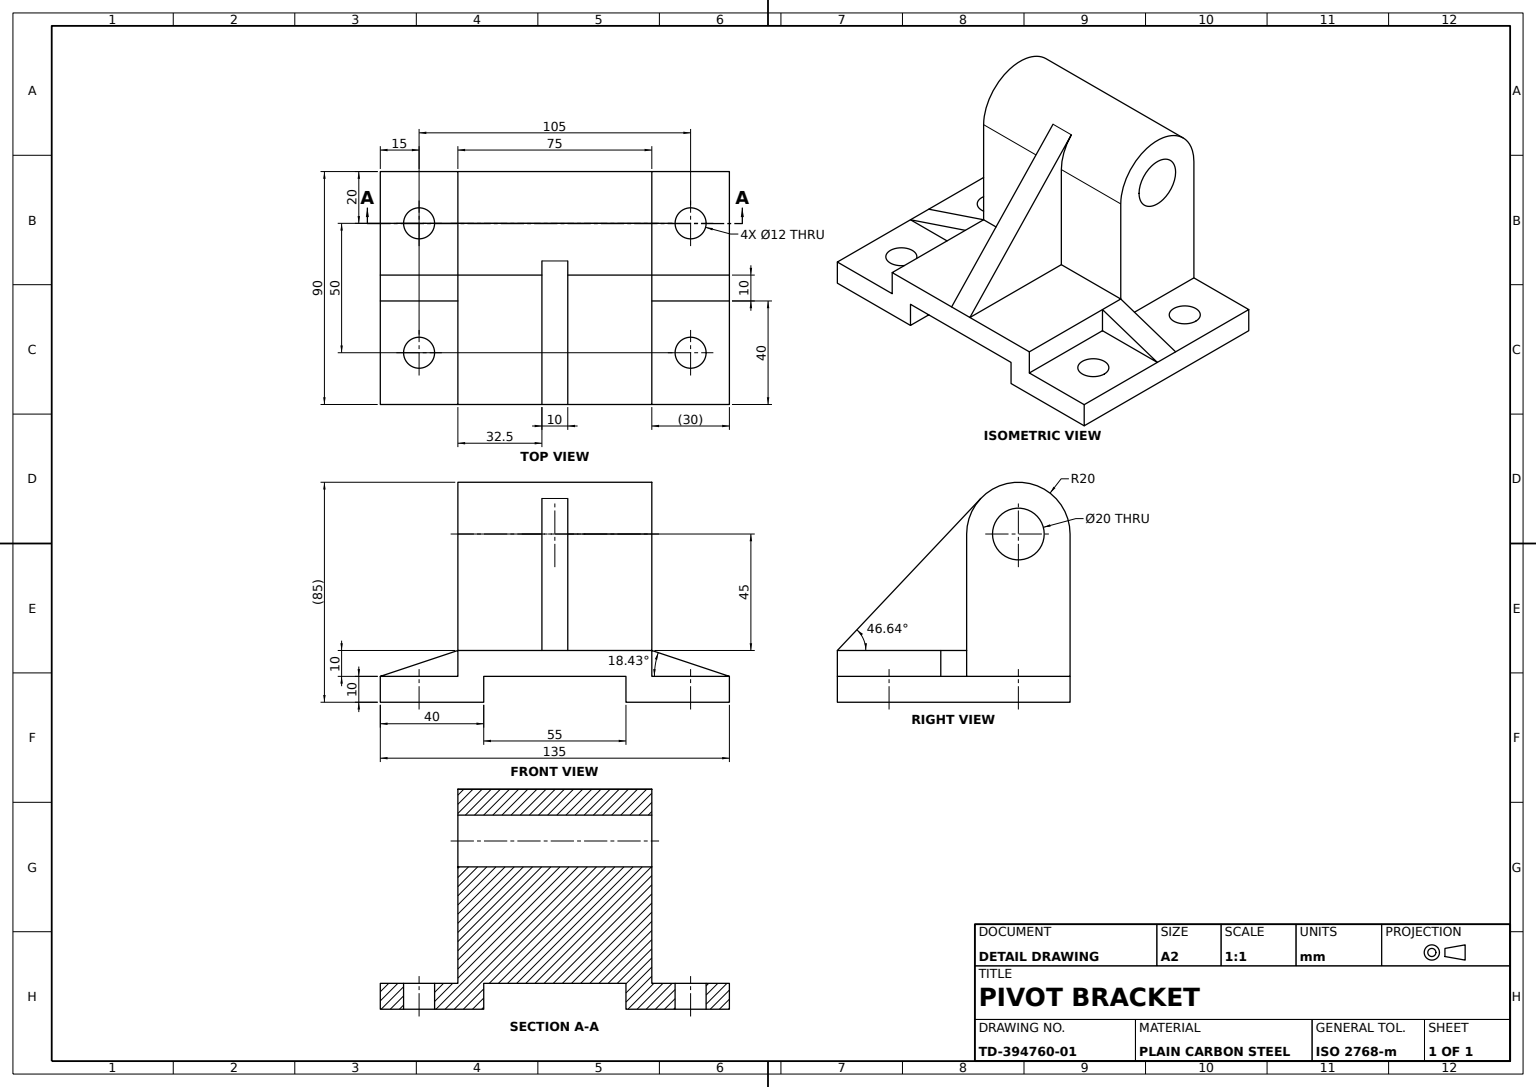
from build123d import *

# Parameters (mm, degrees)
BASE_PLATE_DEPTH            = 45
MOUNTING_HOLES_SKETCH_R     = 6
MOUNTING_HOLES_DEPTH        = 40
PIVOT_BOSS_PROFILE_R        = 10
PIVOT_BOSS_DEPTH            = 75
CENTER_GUSSET_RIB_REACH     = 119.5
CENTER_GUSSET_SKETCH_WALL_W = 317.777472108
CENTER_GUSSET_SKETCH_WALL_H = 10
SIDE_GUSSET_RIB_REACH       = 119.5
SIDE_GUSSET_SKETCH_WALL_W   = 268.622776602
SIDE_GUSSET_SKETCH_WALL_H   = 10


with BuildPart() as part:
    # Base Plate Profile → Base Plate (new, symmetric)
    with BuildSketch(Plane.XY):
        Polygon((-67.5, 0), (-27.5, 0), (-27.5, 10), (27.5, 10), (27.5, 0), (67.5, 0), (67.5, 10), (37.5, 10), (37.5, 20), (-37.5, 20), (-37.5, 10), (-67.5, 10), align=None)
    extrude(amount=BASE_PLATE_DEPTH, both=True)

    # Mounting Holes Sketch → Mounting Holes (cut)
    with BuildSketch(Plane(origin=(0, 10, 0), x_dir=(1, 0, 0), z_dir=(0, 1, 0))):
        with Locations(Location((52.5, -25, 0), (0, 0, 180))):
            Circle(MOUNTING_HOLES_SKETCH_R)
        with Locations(Location((52.5, 25, 0), (0, 0, 180))):
            Circle(MOUNTING_HOLES_SKETCH_R)
        with Locations(Location((-52.5, 25, 0), (0, 0, 270))):
            Circle(MOUNTING_HOLES_SKETCH_R)
        with Locations(Location((-52.5, -25, 0), (0, 0, 270))):
            Circle(MOUNTING_HOLES_SKETCH_R)
    extrude(amount=-MOUNTING_HOLES_DEPTH, mode=Mode.SUBTRACT)

    # Pivot Boss Profile → Pivot Boss (add)
    with BuildSketch(Plane(origin=(37.5, 0, 0), x_dir=(0, 0, -1), z_dir=(1, 0, 0))):
        with BuildLine():
            Line((45, 20), (5, 20))
            Line((5, 20), (5, 65))
            ThreePointArc((5, 65), (25, 85), (45, 65))
            Line((45, 65), (45, 20))
        make_face()
        with Locations((25, 65)):
            Circle(PIVOT_BOSS_PROFILE_R, mode=Mode.SUBTRACT)
    extrude(amount=-PIVOT_BOSS_DEPTH)

    # Center Gusset Sketch wall → Center Gusset Rib (add, up to next)
    with BuildSketch(Plane(origin=(0, 49.365592849, 17.270738259), x_dir=(0, -0.727073825966, 0.686559284837), z_dir=(0, -0.686559284837, -0.727073825966)), mode=Mode.PRIVATE) as center_gusset_rib_sk1:
        Rectangle(CENTER_GUSSET_SKETCH_WALL_W, CENTER_GUSSET_SKETCH_WALL_H)
    center_gusset_rib_tool1 = extrude(center_gusset_rib_sk1.sketch, amount=CENTER_GUSSET_RIB_REACH, mode=Mode.PRIVATE) - part.part
    add(center_gusset_rib_tool1.solids().sort_by_distance((0, 49.365592849, 17.270738259))[0])

    # Side Gusset Sketch wall → Side Gusset Rib (add, up to next)
    with BuildSketch(Plane(origin=(-52.5, 15, 0), x_dir=(-0.948683298051, -0.316227766017, 0), z_dir=(0.316227766017, -0.948683298051, 0)), mode=Mode.PRIVATE) as side_gusset_rib_sk1:
        Rectangle(SIDE_GUSSET_SKETCH_WALL_W, SIDE_GUSSET_SKETCH_WALL_H)
    side_gusset_rib_tool1 = extrude(side_gusset_rib_sk1.sketch, amount=SIDE_GUSSET_RIB_REACH, mode=Mode.PRIVATE) - part.part
    side_gusset_rib = side_gusset_rib_tool1.solids().sort_by_distance((-52.5, 15, 0))[0]
    add(side_gusset_rib)

    # Side Gusset Mirror: Side Gusset Rib across plane
    add(side_gusset_rib.mirror(Plane(origin=(0, 0, 0), x_dir=(0, 0, 1), z_dir=(1, 0, 0))))


solid = part.part
